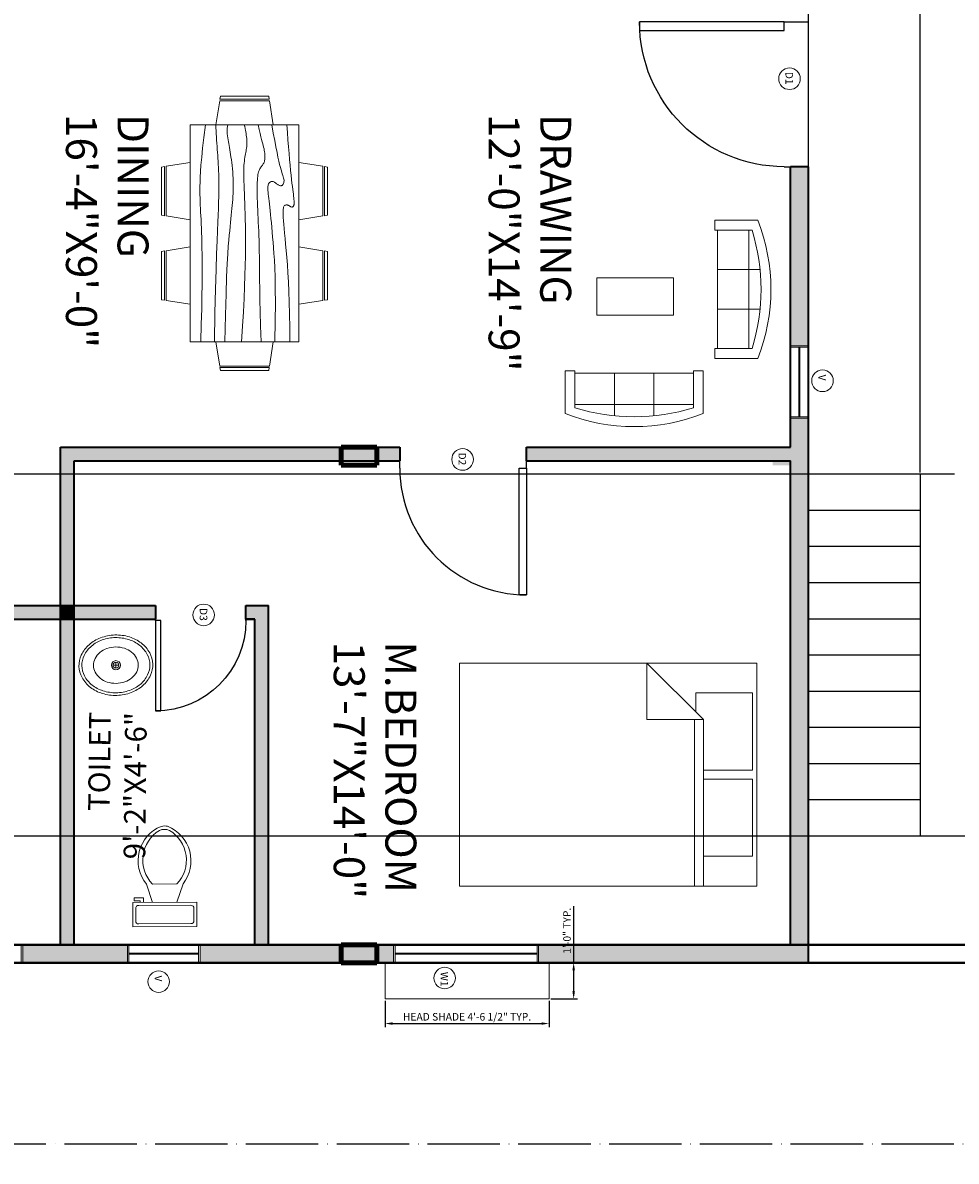
# Model space of a CAD drawing. Units: inches. Extents: x 7028582 to 7030319, y 63109697 to 63111305.
# Tile 5 of 18: x 7029402 to 7029711, y 63109901 to 63110278. Entities that reach past the tile are written whole.
import ezdxf

# ---------------------------------------------------------------- set-up
doc = ezdxf.new("R2010")
doc.units = ezdxf.units.IN
doc.linetypes.add('ACAD_ISO04W100', pattern=[30, 24, -3, 0, -3])
for name, color, linetype, lineweight in [('A-AREA-IDEN', 7, 'Continuous', 18), ('A-DOOR-IDEN', 20, 'Continuous', 13), ('A-FLOR-FIXT', 9, 'Continuous', 18), ('A-FLOR-STRS', 1, 'Continuous', 25), ('A-GLAZ-IDEN', 20, 'Continuous', 13), ('A-WALL-PATT', 8, 'Continuous', 13), ('C-ANNO-DIMS', 7, 'Continuous', 18), ('C-PROP', 1, 'ACAD_ISO04W100', 25), ('doors', 20, 'Continuous', 25), ('furniture', 9, 'Continuous', 18), ('PILLARS', 220, 'Continuous', 100), ('S-COLS-PATT', 220, 'Continuous', 100), ('walls', 6, 'Continuous', 35), ('WINDOW SHADOW', 9, 'Continuous', 13), ('windows', 5, 'Continuous', 18)]:
    doc.layers.add(name, color=color, linetype=linetype, lineweight=lineweight)
doc.styles.get("Standard").update_dxf_attribs({"font": 'arial.ttf'})
doc.dimstyles.new('ISO-25', dxfattribs={"dimtxt": 2.5, "dimasz": 2.5, "dimexe": 1.25, "dimexo": 0.625, "dimtad": 1, "dimlunit": 4, "dimtxsty": 'Standard', "dimcen": 2.5, "dimadec": 0, "dimazin": 0, "dimtfac": 1, "dimtmove": 0, "dimatfit": 3, "dimfxl": 1, "dimarcsym": 0})

# ---------------------------------------------------------------- blocks, each defined once
blk = doc.blocks.new('*U2')
for p, q in [((0, 0), (0, -5)), ((30, 0), (30, -5))]:
    blk.add_line(p, q)
blk.add_lwpolyline([(0, 0), (0, 30), (1.75, 30), (1.75, 0)], close=True)
blk.add_arc((0, 0), 30, 0, 90)
blk = doc.blocks.new('Dining Set - 36 x 72 in.')
for p, q in [((-22, 27.5), (-22.1562, 26.50042)), ((-5.8416, 26.5), (-22.1534, 26.5)), ((-22, 27.5), (-6, 27.5)), ((-5.8437, 26.49966), (-6, 27.5)), ((6, 27.5), (5.8438, 26.50042)), ((22.1584, 26.5), (5.8466, 26.5)), ((6, 27.5), (22, 27.5)), ((22.1563, 26.49966), (22, 27.5)), ((-22.2343, 26.00059), (-23.4847, 17.99762)), ((-22.2304, 26), (-5.7608, 26)), ((-4.5152, 17.99762), (-5.7655, 25.99926)), ((5.7657, 26.00059), (4.5153, 17.99762)), ((5.7696, 26), (22.2392, 26)), ((23.4848, 17.99762), (22.2345, 25.99926)), ((36, 18), (-36, 18)), ((-36, 18), (-36, -18)), ((36, -18), (36, 18)), ((-45.5, 8), (-44.5004, 8.15617)), ((-45.5, 8), (-45.5, -8)), ((-44.5, -8.15843), (-44.5, 8.15338)), ((-44.0006, 8.23428), (-35.9976, 9.48474)), ((-44, 8.23041), (-44, -8.23915)), ((44.0006, 8.23428), (35.9976, 9.48474)), ((44, 8.23041), (44, -8.23915)), ((44.5, -8.15843), (44.5, 8.15338)), ((45.5, 8), (44.5005, 8.15617)), ((45.5, 8), (45.5, -8)), ((-44.4997, -8.15631), (-45.5, -8)), ((-35.9976, -9.48476), (-43.9993, -8.2345)), ((35.9976, -9.48476), (43.9993, -8.2345)), ((44.4997, -8.15631), (45.5, -8)), ((-36, -18), (36, -18)), ((-22.2343, -26.0006), (-23.4847, -17.99762)), ((-4.5152, -17.99762), (-5.7655, -25.99928)), ((5.7657, -26.0006), (4.5153, -17.99762)), ((23.4848, -17.99762), (22.2345, -25.99928)), ((-22.2304, -26), (-5.7608, -26)), ((5.7696, -26), (22.2392, -26)), ((-22, -27.5), (-22.1562, -26.50044)), ((-5.8416, -26.5), (-22.1534, -26.5)), ((-22, -27.5), (-6, -27.5)), ((-5.8437, -26.49967), (-6, -27.5)), ((6, -27.5), (5.8438, -26.50044)), ((22.1584, -26.5), (5.8466, -26.5)), ((6, -27.5), (22, -27.5)), ((22.1563, -26.49967), (22, -27.5))]:
    blk.add_line(p, q)
for points in [[(-36, 15), (-31.1772, 14.97754), (-26.8079, 14.91406), (-22.8538, 14.81543), (-19.276, 14.6875), (-16.0362, 14.53613), (-13.0957, 14.36718), (-10.4159, 14.18652), (-7.9583, 14), (-5.6904, 13.81315), (-3.6035, 13.63021), (-1.6954, 13.45508), (0.0365, 13.29166), (1.5945, 13.14388), (2.9811, 13.01562), (4.1988, 12.9108), (5.25, 12.83333), (6.1393, 12.78613), (6.8802, 12.76823), (7.4883, 12.77767), (7.9792, 12.8125), (8.3685, 12.87077), (8.6719, 12.95052), (8.9049, 13.0498), (9.0833, 13.16666), (9.2205, 13.29899), (9.3216, 13.44401), (9.3895, 13.59879), (9.4271, 13.76041), (9.4373, 13.92594), (9.4232, 14.09245), (9.3875, 14.257), (9.3333, 14.41666), (9.2638, 14.56917), (9.1836, 14.71484), (9.0975, 14.85465), (9.0104, 14.98958), (8.9272, 15.1206), (8.8529, 15.2487), (8.7922, 15.37483), (8.75, 15.5), (8.7305, 15.62467), (8.7344, 15.74739), (8.7617, 15.86621), (8.8125, 15.97916), (8.8867, 16.08431), (8.9844, 16.17968), (9.1055, 16.26334), (9.25, 16.33333), (9.4189, 16.38802), (9.6172, 16.42708), (9.8506, 16.45052), (10.125, 16.45833), (10.4463, 16.45052), (10.8203, 16.42708), (11.2529, 16.38802), (11.75, 16.33333), (12.3184, 16.26318), (12.9694, 16.17838), (13.7151, 16.07991), (14.5677, 15.96875), (15.5395, 15.84586), (16.6426, 15.71224), (17.8893, 15.56884), (19.2917, 15.41666), (20.859, 15.25667), (22.5879, 15.08984), (24.4721, 14.91715), (26.5052, 14.73958), (28.6809, 14.5581), (30.9929, 14.3737), (33.4347, 14.18733), (36, 14)], [(-36, 10), (-28.9766, 10.14274), (-23.1725, 10.20442), (-18.4241, 10.19775), (-14.5677, 10.13541), (-11.4399, 10.03011), (-8.877, 9.89453), (-6.7154, 9.74137), (-4.7917, 9.58333), (-2.9698, 9.43082), (-1.2246, 9.28515), (0.4415, 9.14534), (2.026, 9.01041), (3.5266, 8.87939), (4.9408, 8.7513), (6.266, 8.62516), (7.5, 8.5), (8.6411, 8.37549), (9.6914, 8.2539), (10.6538, 8.13818), (11.5312, 8.03125), (12.3267, 7.93603), (13.043, 7.85547), (13.6831, 7.79248), (14.25, 7.75), (14.7471, 7.7303), (15.1797, 7.73307), (15.5537, 7.75732), (15.875, 7.80208), (16.1494, 7.86637), (16.3828, 7.94922), (16.5811, 8.04964), (16.75, 8.16666), (16.8944, 8.29915), (17.0143, 8.44531), (17.1089, 8.60319), (17.1771, 8.77083), (17.218, 8.94629), (17.2305, 9.1276), (17.2137, 9.31282), (17.1667, 9.5), (17.0895, 9.6875), (16.987, 9.875), (16.8649, 10.0625), (16.7292, 10.25), (16.5856, 10.4375), (16.4401, 10.625), (16.2985, 10.8125), (16.1667, 11), (16.05, 11.18733), (15.9518, 11.3737), (15.8752, 11.5581), (15.8229, 11.73958), (15.798, 11.91715), (15.8034, 12.08984), (15.842, 12.25667), (15.9167, 12.41666), (16.0295, 12.56836), (16.1784, 12.70833), (16.3605, 12.83268), (16.5729, 12.9375), (16.8127, 13.01888), (17.0768, 13.07291), (17.3625, 13.0957), (17.6667, 13.08333), (17.9894, 13.03312), (18.3418, 12.94726), (18.7382, 12.82918), (19.1927, 12.68229), (19.7195, 12.51001), (20.3327, 12.31575), (21.0465, 12.10294), (21.875, 11.875), (22.8357, 11.63354), (23.959, 11.37304), (25.2786, 11.08618), (26.8282, 10.76562), (28.6414, 10.40405), (30.752, 9.99414), (33.1936, 9.52856), (36, 9)], [(-36, 5.5), (-30.7157, 5.3348), (-26.069, 5.20963), (-21.9946, 5.11767), (-18.4271, 5.05208), (-15.3009, 5.00602), (-12.5508, 4.97265), (-10.1112, 4.94515), (-7.9167, 4.91666), (-5.909, 4.88167), (-4.0586, 4.83984), (-2.3429, 4.79215), (-0.7396, 4.73958), (0.7739, 4.6831), (2.22, 4.6237), (3.6213, 4.56233), (5, 4.5), (6.373, 4.43782), (7.7344, 4.3776), (9.0723, 4.32129), (10.375, 4.27083), (11.6309, 4.22819), (12.8281, 4.19531), (13.9551, 4.17415), (15, 4.16666), (15.954, 4.17448), (16.819, 4.19791), (17.6001, 4.23698), (18.3021, 4.29166), (18.9299, 4.36198), (19.4883, 4.44791), (19.9823, 4.54948), (20.4167, 4.66666), (20.7969, 4.79899), (21.1302, 4.94401), (21.4245, 5.09879), (21.6875, 5.26041), (21.9271, 5.42594), (22.1511, 5.59245), (22.3672, 5.757), (22.5834, 5.91666), (22.8065, 6.06868), (23.0404, 6.21093), (23.2879, 6.34147), (23.5521, 6.45833), (23.8358, 6.55957), (24.142, 6.64323), (24.4735, 6.70735), (24.8334, 6.75), (25.2235, 6.76969), (25.642, 6.76692), (26.0858, 6.74267), (26.5521, 6.69791), (27.0379, 6.63362), (27.5404, 6.55078), (28.0565, 6.45036), (28.5834, 6.33333), (29.1242, 6.19987), (29.7071, 6.04687), (30.3661, 5.87044), (31.1354, 5.66666), (32.0493, 5.43164), (33.142, 5.16146), (34.4475, 4.85221), (36, 4.5)], [(-36, -1), (-30.7915, -0.6591), (-26.0195, -0.38216), (-21.6519, -0.16284), (-17.6563, 0.00521), (-14.0005, 0.12833), (-10.6523, 0.21289), (-7.5796, 0.26522), (-4.75, 0.29166), (-2.134, 0.29793), (0.2878, 0.28711), (2.5317, 0.26163), (4.6146, 0.22396), (6.5529, 0.17651), (8.3633, 0.12174), (10.0623, 0.06209), (11.6667, 0), (13.1899, -0.06201), (14.6341, -0.1211), (15.9982, -0.17432), (17.2813, -0.21875), (18.4823, -0.25147), (19.6003, -0.26953), (20.6343, -0.27002), (21.5834, -0.25), (22.4481, -0.20768), (23.2357, -0.14584), (23.9549, -0.06836), (24.6146, 0.02083), (25.2235, 0.11784), (25.7904, 0.21875), (26.3241, 0.31966), (26.8334, 0.41666), (27.3265, 0.50618), (27.8099, 0.58593), (28.2894, 0.65397), (28.7709, 0.70833), (29.2601, 0.74707), (29.763, 0.76823), (30.2855, 0.76985), (30.8334, 0.75), (31.4088, 0.70784), (31.9994, 0.64713), (32.589, 0.57275), (33.1615, 0.48958), (33.7008, 0.4025), (34.1908, 0.3164), (34.6153, 0.23616), (34.9584, 0.16666), (35.2099, 0.11165), (35.3848, 0.07031), (35.504, 0.04069), (35.5886, 0.02083), (35.6594, 0.00879), (35.7377, 0.0026), (35.8442, 0.00032), (36, 0)], [(-36, -6.5), (-27.1843, -6.31267), (-20.084, -6.1263), (-14.469, -5.9419), (-10.1094, -5.76042), (-6.7752, -5.58285), (-4.2363, -5.41016), (-2.2629, -5.24333), (-0.625, -5.08334), (0.8708, -4.93099), (2.2715, -4.78646), (3.5872, -4.64974), (4.8281, -4.52084), (6.0046, -4.39974), (7.127, -4.28646), (8.2053, -4.18099), (9.25, -4.08334), (10.2705, -3.99382), (11.2734, -3.91407), (12.2647, -3.84603), (13.25, -3.79167), (14.2354, -3.75293), (15.2266, -3.73177), (16.2295, -3.73015), (17.25, -3.75), (18.2912, -3.79248), (19.3451, -3.85547), (20.4009, -3.93604), (21.4479, -4.03125), (22.4754, -4.13819), (23.4727, -4.25391), (24.4289, -4.37549), (25.3334, -4.5), (26.1785, -4.62492), (26.9694, -4.74935), (27.7145, -4.87281), (28.4219, -4.99479), (29.1, -5.11483), (29.7572, -5.23242), (30.4016, -5.34709), (31.0417, -5.45834), (31.6837, -5.56437), (32.3262, -5.65821), (32.9658, -5.73153), (33.599, -5.77604), (34.2224, -5.78345), (34.8327, -5.74545), (35.4264, -5.65373), (36, -5.5)], [(-36, -10), (-26.4022, -9.81299), (-18.4675, -9.62891), (-11.9839, -9.45069), (-6.7396, -9.28125), (-2.5226, -9.12354), (0.8789, -8.98047), (3.6769, -8.85498), (6.0833, -8.75), (8.2767, -8.66765), (10.3021, -8.60677), (12.1712, -8.56543), (13.8958, -8.54167), (15.4876, -8.53353), (16.9583, -8.53907), (18.3197, -8.55632), (19.5834, -8.58334), (20.7616, -8.61841), (21.8685, -8.66081), (22.9188, -8.71004), (23.9271, -8.76563), (24.9081, -8.82707), (25.8763, -8.89388), (26.8465, -8.96558), (27.8334, -9.04167), (28.8474, -9.12118), (29.8828, -9.20117), (30.93, -9.27824), (31.9792, -9.34896), (33.0205, -9.40991), (34.0443, -9.45768), (35.0407, -9.48885), (36, -9.5)], [(-36, -14.5), (-30.0881, -14.33513), (-25.0332, -14.21224), (-20.7312, -14.12647), (-17.0781, -14.07292), (-13.97, -14.04671), (-11.3027, -14.04297), (-8.9724, -14.05681), (-6.875, -14.08334), (-4.9224, -14.11833), (-3.0905, -14.16016), (-1.3709, -14.20785), (0.2448, -14.26042), (1.7647, -14.3169), (3.1973, -14.3763), (4.5507, -14.43767), (5.8333, -14.5), (7.0554, -14.5621), (8.235, -14.62175), (9.3922, -14.67652), (10.5469, -14.72396), (11.7192, -14.76164), (12.929, -14.78711), (14.1965, -14.79794), (15.5417, -14.79167), (16.9933, -14.76424), (18.6152, -14.70508), (20.4804, -14.60197), (22.6615, -14.44271), (25.2312, -14.21509), (28.2624, -13.9069), (31.8277, -13.50594), (36, -13)]]:
    blk.add_lwpolyline(points)
blk = doc.blocks.new('Sofa - Roundback 7 ft.')
for p, q in [((-12.00002, -32.4421), (-12.00003, -6.5971)), ((11.99997, -32.4421), (11.99998, -6.5971)), ((-36.000027, -34), (-36.000027, -11.4696)), ((-35.999844, -13.3819), (35.9998, -13.3819)), ((35.99998, -34), (35.99998, -11.4696)), ((-36.000027, -32.4421), (35.99998, -32.4421))]:
    blk.add_line(p, q)
for points in [[(-36.000027, -34), (-42.000027, -34), (-42.000027, -8)], [(41.99998, -8), (41.99998, -34), (35.99998, -34)]]:
    blk.add_lwpolyline(points)
for centre, radius, start, end in [((0, -114.25), 114.25, 68.43141, 111.5686), ((-0.00001, -127.1968), 121.1968, 72.72033, 107.2797)]:
    blk.add_arc(centre, radius, start, end)
blk = doc.blocks.new('Toilet - top')
for p, q in [((9.5, -6), (9.5, -2)), ((-10, -8.5), (-8, -8.5)), ((-10, -9.5), (-10, -8.5)), ((-7, -9.5), (-10, -9.5)), ((-8, -8.5), (-8, -8)), ((-7, -8), (-7, -9.5)), ((-4, -8), (-6, -14)), ((4, -8), (6, -14)), ((4, -14), (-4, -14))]:
    blk.add_line(p, q)
blk.add_lwpolyline([(10.5, -8), (10.5, 0), (-10.5, 0), (-10.5, -8)], close=True)
for points in [[(-9.5, -2), (-9.5, -6)], [(8.5, -1), (-8.5, -1)], [(-8.5, -7), (8.5, -7)]]:
    blk.add_lwpolyline(points)
for centre, radius, start, end in [((-8.62, -1.88), 0.884, 81.8699, 188.1301), ((8.62, -1.88), 0.884, 351.8699, 98.1301), ((-8.62, -6.12), 0.884, 171.8699, 278.1301), ((8.62, -6.12), 0.884, 261.8699, 8.1301), ((3.52, -21.58), 12.17, 141.4691, 247.9714), ((4.2, -21.82), 11.33, 136.3677, 238.9468), ((-3.52, -21.58), 12.17, 292.0284, 38.5307), ((-4.2, -21.82), 11.33, 301.053, 43.6321), ((0, -27.88), 4, 245.7318, 294.2682), ((0, -29), 4, 254.8605, 285.1395)]:
    blk.add_arc(centre, radius, start, end)
blk = doc.blocks.new('Sink - Oval top')
for p, q in [((-1, 0), (1, 0)), ((0, 1), (0, -1))]:
    blk.add_line(p, q)
for points in [[(-12.23, 0.39, 0.117634), (-11.46, -3.36, 0.104469), (-8.88, -6.8, 0.090016), (-5.08, -9.07, 0.08192), (-0.32, -10.02, 0.08192), (4.49, -9.38, 0.090016), (8.42, -7.36, 0.104469), (11.22, -4.09, 0.117634), (12.23, -0.39, 0.117634), (11.46, 3.36, 0.104469), (8.88, 6.8, 0.090016), (5.08, 9.07, 0.08192), (0.32, 10.02, 0.08192), (-4.49, 9.38, 0.090016), (-8.42, 7.36, 0.104469), (-11.22, 4.09, 0.117634)], [(-11.29, 0.16, 0.118622), (-10.52, -3.25, 0.104678), (-8.07, -6.36, 0.089562), (-4.54, -8.37, 0.081185), (-0.13, -9.15, 0.081185), (4.3, -8.49, 0.089562), (7.89, -6.58, 0.104678), (10.42, -3.55, 0.118622), (11.29, -0.16, 0.118622), (10.52, 3.25, 0.104678), (8.07, 6.36, 0.089562), (4.54, 8.37, 0.081185), (0.13, 9.15, 0.081185), (-4.3, 8.49, 0.089562), (-7.89, 6.58, 0.104678), (-10.42, 3.55, 0.118622)], [(-7.42, 0.08, 0.118283), (-6.91, -2.17, 0.104607), (-5.29, -4.21, 0.089718), (-2.97, -5.53, 0.081436), (-0.07, -6.04, 0.081436), (2.84, -5.59, 0.089718), (5.2, -4.33, 0.104607), (6.86, -2.32, 0.118283), (7.42, -0.08, 0.118283), (6.91, 2.17, 0.104607), (5.29, 4.21, 0.089718), (2.97, 5.53, 0.081436), (0.07, 6.04, 0.081436), (-2.84, 5.59, 0.089718), (-5.2, 4.33, 0.104607), (-6.86, 2.32, 0.118283)]]:
    blk.add_lwpolyline(points, format="xyb", close=True)
for radius in [1.5, 1]:
    blk.add_circle((0, 0), radius)
blk = doc.blocks.new('Bed - Queen')
for p, q in [((0, -80.00003), (0, 0)), ((0, 0), (59.99999, 0)), ((59.99999, 0), (59.99999, -80.00003)), ((7.99999, -1.2), (28.79998, -1.2)), ((7.99999, -14.4), (7.99999, -1.2)), ((28.79998, -1.2), (28.79998, -14.4)), ((31.19999, -1.2), (51.99999, -1.2)), ((31.19999, -14.4), (31.19999, -1.2)), ((51.99999, -1.2), (51.99999, -16.4)), ((0, -14.4), (44.8, -14.4)), ((59.99999, -29.6), (44.8, -14.4)), ((44.8, -14.4), (44.8, -29.6)), ((44.8, -16.8), (0, -16.8)), ((51.99999, -16.4), (46.79936, -16.4)), ((44.8, -29.6), (59.99999, -29.6)), ((59.99999, -80.00003), (0, -80.00003))]:
    blk.add_line(p, q)
blk = doc.blocks.new('WIN-SASH-24')
for p, q in [((24.05, 6), (0, 6)), ((0.5, 6), (0.5, 0)), ((23.55, 0), (23.55, 6)), ((0, 0), (24.05, 0)), ((23.55, 3.2), (0.5, 3.2)), ((23.55, 2.8), (0.5, 2.8))]:
    blk.add_line(p, q)
blk = doc.blocks.new('WIN-SASH-24-FRAME')
for p, q in [((24.05, 6), (0, 6)), ((0.5, 6), (0.5, 0)), ((23.55, 0), (23.55, 6)), ((0, 0), (24.05, 0))]:
    blk.add_line(p, q)
blk = doc.blocks.new('WIN-SASH-48')
for p, q in [((48.05, 6), (0, 6)), ((0.5, 6), (0.5, 0)), ((47.55, 0), (47.55, 6)), ((47.55, 3.2), (0.5, 3.2)), ((47.55, 2.8), (0.5, 2.8)), ((0, 0), (48.05, 0))]:
    blk.add_line(p, q)
blk = doc.blocks.new('WINDOW-SHADE-HEAD-54')
for p, q in [((0, 0), (0, 12)), ((54.39, 12), (54.39, 0)), ((54.39, 0), (0, 0))]:
    blk.add_line(p, q)
blk = doc.blocks.new('COLUMN-RECT-PROFILE')
for p, q in [((11.91, 6), (0, 6)), ((0, 6), (0, 0)), ((11.91, 0), (11.91, 6)), ((0, 0), (11.91, 0))]:
    blk.add_line(p, q)
blk = doc.blocks.new('TABLE-COFFEE-RECT')
blk.add_lwpolyline([(25.34, 12.34), (0, 12.34), (0, 0), (25.34, 0)], close=True)
blk = doc.blocks.new('TAG-D2-ST-L')
blk.add_circle((3.58, 3.58), 3.58)
blk.add_text('D2', height=2.5, rotation=270).set_placement((2.23, 5.87))
blk = doc.blocks.new('TAG-D3-ST-L')
blk.add_circle((3.58, 3.58), 3.58)
blk.add_text('D3', height=2.5, rotation=270).set_placement((2.27, 5.87))
blk = doc.blocks.new('TAG-V-ST-L')
blk.add_circle((3.58, 3.58), 3.58)
blk.add_text('V', height=2.5, rotation=270).set_placement((2.23, 5.62))
blk = doc.blocks.new('TAG-W1-ST-L')
blk.add_circle((3.58, 3.58), 3.58)
blk.add_text('W1', height=2.5, rotation=270).set_placement((2.23, 5.64))
blk = doc.blocks.new('*D93')
at = {"layer": 'C-ANNO-DIMS', "color": 0, "lineweight": -2, "transparency": 16777216}
for p, q in [((7029521.82, 63109953.93), (7029521.82, 63109945.15)), ((7029576.21, 63109953.93), (7029576.21, 63109945.15)), ((7029524.32, 63109946.4), (7029573.71, 63109946.4))]:
    blk.add_line(p, q, dxfattribs=at)
at = {"layer": 'C-ANNO-DIMS', "color": 0, "lineweight": 100, "transparency": 16777216}
for points in [[(7029524.32, 63109946.81), (7029524.32, 63109945.98), (7029521.82, 63109946.4)], [(7029573.71, 63109946.81), (7029573.71, 63109945.98), (7029576.21, 63109946.4)]]:
    blk.add_solid(points, dxfattribs=at)
at = {"layer": 'Defpoints', "color": 0, "lineweight": 100, "transparency": 16777216}
for p in [(7029521.82, 63109954.56), (7029576.21, 63109954.56), (7029576.21, 63109946.4)]:
    blk.add_point(p, dxfattribs=at)
at = {"layer": 'C-ANNO-DIMS', "color": 0, "transparency": 16777216, "insert": (7029549.01, 63109948.32), "char_height": 2.5, "attachment_point": 5}
blk.add_mtext('HEAD SHADE 4\'-6 1/2" TYP.', dxfattribs=at)
blk = doc.blocks.new('*D94')
at = {"layer": 'C-ANNO-DIMS', "color": 0, "lineweight": -2, "transparency": 16777216}
for p, q in [((7029584.37, 63109966.56), (7029584.37, 63109985.31)), ((7029576.84, 63109966.56), (7029585.62, 63109966.56)), ((7029584.37, 63109957.06), (7029584.37, 63109964.06)), ((7029576.84, 63109954.56), (7029585.62, 63109954.56))]:
    blk.add_line(p, q, dxfattribs=at)
at = {"layer": 'C-ANNO-DIMS', "color": 0, "lineweight": 100, "transparency": 16777216}
for points in [[(7029583.95, 63109964.06), (7029584.79, 63109964.06), (7029584.37, 63109966.56)], [(7029583.95, 63109957.06), (7029584.79, 63109957.06), (7029584.37, 63109954.56)]]:
    blk.add_solid(points, dxfattribs=at)
at = {"layer": 'Defpoints', "color": 0, "lineweight": 100, "transparency": 16777216}
for p in [(7029576.21, 63109966.56), (7029584.37, 63109966.56), (7029576.21, 63109954.56)]:
    blk.add_point(p, dxfattribs=at)
at = {"layer": 'C-ANNO-DIMS', "color": 0, "transparency": 16777216, "insert": (7029582.47, 63109977.18), "char_height": 2.5, "attachment_point": 5, "rotation": 90}
blk.add_mtext('1\'-0" TYP.', dxfattribs=at)
blk = doc.blocks.new('*D99')
at = {"layer": 'C-ANNO-DIMS', "color": 0, "lineweight": -2, "transparency": 16777216}
for p, q in [((7029234.71, 63109965.93), (7029234.71, 63109697.14)), ((7030175.71, 63109965.93), (7030175.71, 63109697.14)), ((7029237.21, 63109698.39), (7030173.21, 63109698.39))]:
    blk.add_line(p, q, dxfattribs=at)
at = {"layer": 'C-ANNO-DIMS', "color": 0, "lineweight": 100, "transparency": 16777216}
for points in [[(7029237.21, 63109698.8), (7029237.21, 63109697.97), (7029234.71, 63109698.39)], [(7030173.21, 63109698.8), (7030173.21, 63109697.97), (7030175.71, 63109698.39)]]:
    blk.add_solid(points, dxfattribs=at)
at = {"layer": 'Defpoints', "color": 0, "lineweight": 100, "transparency": 16777216}
for p in [(7029234.71, 63109966.56), (7030175.71, 63109966.56), (7030175.71, 63109698.39)]:
    blk.add_point(p, dxfattribs=at)
at = {"layer": 'C-ANNO-DIMS', "color": 0, "transparency": 16777216, "insert": (7029705.21, 63109700.29), "char_height": 2.5, "attachment_point": 5}
blk.add_mtext('78\'-5"', dxfattribs=at)
blk = doc.blocks.new('*D108')
at = {"layer": 'C-ANNO-DIMS', "color": 0, "lineweight": -2, "transparency": 16777216}
for p, q in [((7029662.21, 63110129.18), (7029662.21, 63111300.44)), ((7029664.71, 63111299.19), (7029696.71, 63111299.19)), ((7029699.21, 63110129.18), (7029699.21, 63111300.44))]:
    blk.add_line(p, q, dxfattribs=at)
at = {"layer": 'C-ANNO-DIMS', "color": 0, "lineweight": 100, "transparency": 16777216}
for points in [[(7029664.71, 63111299.61), (7029664.71, 63111298.77), (7029662.21, 63111299.19)], [(7029696.71, 63111299.61), (7029696.71, 63111298.77), (7029699.21, 63111299.19)]]:
    blk.add_solid(points, dxfattribs=at)
at = {"layer": 'Defpoints', "color": 0, "lineweight": 100, "transparency": 16777216}
for p in [(7029699.21, 63111299.19), (7029662.21, 63110128.56), (7029699.21, 63110128.56)]:
    blk.add_point(p, dxfattribs=at)
at = {"layer": 'C-ANNO-DIMS', "color": 0, "transparency": 16777216, "insert": (7029680.71, 63111301.09), "char_height": 2.5, "attachment_point": 5}
blk.add_mtext('3\'-1"', dxfattribs=at)
blk = doc.blocks.new('*D109')
at = {"layer": 'C-ANNO-DIMS', "color": 0, "lineweight": -2, "transparency": 16777216}
for p, q in [((7029710.58, 63110128.56), (7028586.23, 63110128.56)), ((7028587.48, 63110126.06), (7028587.48, 63110011.06)), ((7029710.58, 63110008.56), (7028586.23, 63110008.56))]:
    blk.add_line(p, q, dxfattribs=at)
at = {"layer": 'C-ANNO-DIMS', "color": 0, "lineweight": 100, "transparency": 16777216}
for points in [[(7028587.06, 63110126.06), (7028587.89, 63110126.06), (7028587.48, 63110128.56)], [(7028587.06, 63110011.06), (7028587.89, 63110011.06), (7028587.48, 63110008.56)]]:
    blk.add_solid(points, dxfattribs=at)
at = {"layer": 'Defpoints', "color": 0, "lineweight": 100, "transparency": 16777216}
for p in [(7029711.21, 63110128.56), (7028587.48, 63110008.56), (7029711.21, 63110008.56)]:
    blk.add_point(p, dxfattribs=at)
at = {"layer": 'C-ANNO-DIMS', "color": 0, "transparency": 16777216, "insert": (7028585.57, 63110068.56), "char_height": 2.5, "attachment_point": 5, "rotation": 90}
blk.add_mtext('10\'-0"', dxfattribs=at)
blk = doc.blocks.new('*D110')
at = {"layer": 'C-ANNO-DIMS', "color": 0, "lineweight": -2, "transparency": 16777216}
for p, q in [((7029747.58, 63110008.56), (7028586.23, 63110008.56)), ((7028587.48, 63110006.06), (7028587.48, 63109975.06)), ((7029747.58, 63109972.56), (7028586.23, 63109972.56))]:
    blk.add_line(p, q, dxfattribs=at)
at = {"layer": 'C-ANNO-DIMS', "color": 0, "lineweight": 100, "transparency": 16777216}
for points in [[(7028587.06, 63110006.06), (7028587.89, 63110006.06), (7028587.48, 63110008.56)], [(7028587.06, 63109975.06), (7028587.89, 63109975.06), (7028587.48, 63109972.56)]]:
    blk.add_solid(points, dxfattribs=at)
at = {"layer": 'Defpoints', "color": 0, "lineweight": 100, "transparency": 16777216}
for p in [(7029748.21, 63110008.56), (7028587.48, 63109972.56), (7029748.21, 63109972.56)]:
    blk.add_point(p, dxfattribs=at)
at = {"layer": 'C-ANNO-DIMS', "color": 0, "transparency": 16777216, "insert": (7028585.57, 63109990.56), "char_height": 2.5, "attachment_point": 5, "rotation": 90}
blk.add_mtext('3\'-0"', dxfattribs=at)

msp = doc.modelspace()

# ---------------------------------------------------------------- hatches: boundary and pattern name
at = {"layer": 'A-WALL-PATT'}
h = msp.add_hatch(color=256, dxfattribs=at)
h.dxf.hatch_style = 1
h.paths.add_polyline_path([(7029656.205, 63110230.557), (7029662.205, 63110230.557), (7029662.205, 63110171.186), (7029656.205, 63110171.186)])
h = msp.add_hatch(color=256, dxfattribs=at)
h.dxf.hatch_style = 1
h.paths.add_polyline_path([(7029568.726, 63110137.557), (7029656.205, 63110137.557), (7029656.205, 63110147.137), (7029662.205, 63110147.137), (7029662.205, 63109966.557), (7029572.732, 63109966.557), (7029572.732, 63109972.557), (7029656.205, 63109972.557), (7029656.205, 63110133.057), (7029568.726, 63110133.057)])
h = msp.add_hatch(color=256, dxfattribs=at)
h.dxf.hatch_style = 1
h.paths.add_polyline_path([(7029414.205, 63110137.557), (7029414.205, 63110085.057), (7029418.705, 63110085.057), (7029418.705, 63110133.057), (7029526.726, 63110133.057), (7029526.726, 63110137.557)])
h = msp.add_hatch(color=256, dxfattribs=at)
h.dxf.hatch_style = 1
h.paths.add_polyline_path([(7029414.205, 63110080.557), (7029414.205, 63110085.057), (7029360.705, 63110085.057), (7029360.705, 63110077.557), (7029365.205, 63110077.557), (7029365.205, 63110080.557)])
h = msp.add_hatch(color=256, dxfattribs=at)
h.dxf.hatch_style = 1
h.paths.add_polyline_path([(7029414.205, 63110085.057), (7029418.705, 63110085.057), (7029418.705, 63110080.557), (7029414.205, 63110080.557)])
h = msp.add_hatch(color=256, dxfattribs=at)
h.dxf.hatch_style = 1
h.paths.add_polyline_path([(7029418.705, 63110085.057), (7029445.705, 63110085.057), (7029445.705, 63110080.557), (7029418.705, 63110080.557)])
h = msp.add_hatch(color=256, dxfattribs=at)
h.dxf.hatch_style = 1
h.paths.add_polyline_path([(7029460.479, 63109972.557), (7029478.705, 63109972.557), (7029478.705, 63110080.557), (7029475.705, 63110080.557), (7029475.705, 63110085.057), (7029483.205, 63110085.057), (7029483.205, 63109972.557), (7029524.683, 63109972.557), (7029524.683, 63109966.557), (7029460.479, 63109966.557)])
h = msp.add_hatch(color=256, dxfattribs=at)
h.dxf.hatch_style = 1
h.paths.add_polyline_path([(7029414.205, 63110080.557), (7029414.205, 63109972.557), (7029401.714, 63109972.557), (7029401.714, 63109966.557), (7029436.431, 63109966.557), (7029436.431, 63109972.557), (7029418.705, 63109972.557), (7029418.705, 63110080.557)])
at = {"layer": 'S-COLS-PATT'}
h = msp.add_hatch(color=256, dxfattribs=at)
h.dxf.hatch_style = 1
h.paths.add_polyline_path([(7029662.205, 63110137.557), (7029650.291, 63110137.557), (7029650.291, 63110131.557), (7029662.205, 63110131.557)])
h = msp.add_hatch(color=256, dxfattribs=at)
h.dxf.hatch_style = 1
h.paths.add_polyline_path([(7029662.205, 63109972.505), (7029650.291, 63109972.505), (7029650.291, 63109966.505), (7029662.205, 63109966.505)])

# ---------------------------------------------------------------- linework, layer by layer
at = {"layer": 'A-DOOR-IDEN'}
msp.add_circle((7029655.936, 63110259.719), 3.577, dxfattribs=at)
at = {"layer": 'A-FLOR-STRS'}
for p, q in [((7029662.205, 63110128.557), (7029662.205, 63109972.557)), ((7029699.205, 63110128.557), (7029662.205, 63110128.557)), ((7029699.205, 63110128.557), (7029699.205, 63110008.557)), ((7029699.205, 63110116.557), (7029662.205, 63110116.557)), ((7029699.205, 63110104.557), (7029662.205, 63110104.557)), ((7029699.205, 63110092.557), (7029662.205, 63110092.557)), ((7029699.205, 63110080.557), (7029662.205, 63110080.557)), ((7029699.205, 63110068.557), (7029662.205, 63110068.557)), ((7029699.205, 63110056.557), (7029662.205, 63110056.557)), ((7029699.205, 63110044.557), (7029662.205, 63110044.557)), ((7029699.205, 63110032.557), (7029662.205, 63110032.557)), ((7029699.205, 63110020.557), (7029662.205, 63110020.557)), ((7029748.205, 63110008.557), (7029662.205, 63110008.557))]:
    msp.add_line(p, q, dxfattribs=at)
at = {"layer": 'C-PROP'}
msp.add_line((7029174.705, 63109906.557), (7030235.705, 63109906.557), dxfattribs=at)
at = {"layer": 'walls'}
for p, q in [((7029656.205, 63110137.557), (7029656.205, 63110230.557)), ((7029662.205, 63110230.557), (7029656.205, 63110230.557)), ((7029662.205, 63109966.557), (7029662.205, 63110230.557)), ((7029414.205, 63109972.557), (7029414.205, 63110137.557)), ((7029414.205, 63110137.557), (7029526.726, 63110137.557)), ((7029526.726, 63110137.557), (7029526.726, 63110133.057)), ((7029568.726, 63110137.557), (7029656.205, 63110137.557)), ((7029568.726, 63110133.057), (7029568.726, 63110137.557)), ((7029418.705, 63109972.557), (7029418.705, 63110133.057)), ((7029418.705, 63110133.057), (7029526.726, 63110133.057)), ((7029568.726, 63110133.057), (7029656.205, 63110133.057)), ((7029656.205, 63109972.557), (7029656.205, 63110133.057)), ((7029360.705, 63110085.057), (7029445.705, 63110085.057)), ((7029445.705, 63110085.057), (7029445.705, 63110080.557)), ((7029475.705, 63110085.057), (7029483.205, 63110085.057)), ((7029475.705, 63110080.557), (7029475.705, 63110085.057)), ((7029483.205, 63109972.557), (7029483.205, 63110085.057)), ((7029365.205, 63110080.557), (7029445.705, 63110080.557)), ((7029475.705, 63110080.557), (7029478.705, 63110080.557)), ((7029478.705, 63110080.557), (7029475.705, 63110080.557)), ((7029478.705, 63109972.557), (7029478.705, 63110080.557)), ((7029240.705, 63109972.557), (7030169.705, 63109972.557)), ((7030169.705, 63109972.557), (7029240.705, 63109972.557)), ((7029365.205, 63109972.557), (7029414.205, 63109972.557)), ((7029418.705, 63109972.557), (7029478.705, 63109972.557)), ((7029483.205, 63109972.557), (7029656.205, 63109972.557)), ((7029748.205, 63109972.557), (7029662.205, 63109972.557)), ((7029748.205, 63109972.557), (7029662.205, 63109972.557)), ((7029234.705, 63109966.557), (7030175.705, 63109966.557)), ((7030175.705, 63109966.557), (7029234.705, 63109966.557)), ((7029234.705, 63109966.557), (7029662.205, 63109966.557))]:
    msp.add_line(p, q, dxfattribs=at)
at = {"layer": 'windows'}
for p, q in [((7029656.205, 63110171.186), (7029662.205, 63110171.186)), ((7029662.205, 63110147.137), (7029656.205, 63110147.137)), ((7029401.714, 63109972.557), (7029401.714, 63109966.557)), ((7029436.431, 63109966.557), (7029436.431, 63109972.557)), ((7029460.479, 63109972.557), (7029460.479, 63109966.557)), ((7029524.683, 63109966.557), (7029524.683, 63109972.557)), ((7029572.732, 63109972.557), (7029572.732, 63109966.557))]:
    msp.add_line(p, q, dxfattribs=at)

# ---------------------------------------------------------------- block references
at = {"layer": 'A-DOOR-IDEN'}
for name, p in [('TAG-D2-ST-L', (7029543.956, 63110129.893)), ('TAG-D3-ST-L', (7029458.118, 63110078.328))]:
    msp.add_blockref(name, p, dxfattribs=at)
at = {"layer": 'A-FLOR-FIXT', "xscale": -1}
msp.add_blockref('Sink - Oval top', (7029432.582, 63110065.243), dxfattribs=at)
at = {"layer": 'A-FLOR-FIXT', "xscale": -1.013555723357934, "yscale": 1.013555723357934, "zscale": 1.013555723357934, "rotation": 180.274620379553}
msp.add_blockref('Toilet - top', (7029448.831, 63109978.497), dxfattribs=at)
at = {"layer": 'A-GLAZ-IDEN'}
for name, p in [('TAG-V-ST-L', (7029663.285, 63110155.979)), ('TAG-W1-ST-L', (7029538.009, 63109957.914)), ('TAG-V-ST-L', (7029443.2, 63109956.713))]:
    msp.add_blockref(name, p, dxfattribs=at)
at = {"layer": 'doors'}
for p, xscale, yscale, zscale, rotation in [((7029654.205, 63110278.557), -1.599999999999999, 1.599999999999999, 1.599999999999999, 90), ((7029568.726, 63110130.557), 1.399999999999999, 1.399999999999999, 1.399999999999999, 180)]:
    msp.add_blockref('*U2', p, dxfattribs=dict(at, xscale=xscale, yscale=yscale, zscale=zscale, rotation=rotation))
at = {"layer": 'doors', "xscale": -1, "rotation": 180}
msp.add_blockref('*U2', (7029445.705, 63110080.057), dxfattribs=at)
at = {"layer": 'furniture', "xscale": -1, "rotation": 270}
msp.add_blockref('Dining Set - 36 x 72 in.', (7029475.247, 63110208.448), dxfattribs=at)
at = {"layer": 'furniture'}
for name, p, xscale, yscale, zscale, rotation in [('Sofa - Roundback 7 ft.', (7029649.752, 63110189.875), -0.5455524879488546, 0.5455524879488546, 0.5455524879488546, 270), ('Sofa - Roundback 7 ft.', (7029604.428, 63110144.346), -0.5455524879488546, 0.5455524879488546, 0.5455524879488546, 180), ('Bed - Queen', (7029645.108, 63109992.002), -1.232093012797833, 1.232093012797833, 1.232093012797833, 270)]:
    msp.add_blockref(name, p, dxfattribs=dict(at, xscale=xscale, yscale=yscale, zscale=zscale, rotation=rotation))
at = {"layer": 'furniture', "extrusion": (0, 0, -1), "zscale": -1}
msp.add_blockref('TABLE-COFFEE-RECT', (-7029617.436, 63110181.346), dxfattribs=at)
at = {"layer": 'PILLARS'}
for p in [(7029507.238, 63110131.557), (7029507.238, 63109966.505)]:
    msp.add_blockref('COLUMN-RECT-PROFILE', p, dxfattribs=at)
at = {"layer": 'WINDOW SHADOW'}
msp.add_blockref('WINDOW-SHADE-HEAD-54', (7029521.817, 63109954.557), dxfattribs=at)
at = {"layer": 'windows', "rotation": 269.9999999843229}
msp.add_blockref('WIN-SASH-24', (7029656.205, 63110171.186), dxfattribs=at)
at = {"layer": 'windows'}
for name, p in [('WIN-SASH-24-FRAME', (7029377.666, 63109966.557)), ('WIN-SASH-24', (7029436.431, 63109966.557)), ('WIN-SASH-48', (7029524.683, 63109966.557))]:
    msp.add_blockref(name, p, dxfattribs=at)

# ---------------------------------------------------------------- texts
at = {"layer": 'A-AREA-IDEN'}
for s, width, gutter_width, insert, char_height, attachment_point, rotation in [('DINING\\P16\'-4"X9\'-0"', 82.04322, 51.315, (7029416.035, 63110248.03), 10.26307, 7, 270), ('DRAWING\\P12\'-0"X14\'-9"', 82.04322, 51.315, (7029556.17, 63110248.03), 10.26307, 7, 270), ('M.BEDROOM\\P13\'-7"X14\'-0"', 82.04322, 51.315, (7029504.833, 63110073.083), 10.26307, 7, 270), ('TOILET\\P9\'-2"X4\'-6"', 42.97461, 35.821, (7029423.746, 63110049.835), 7.16426, 3, 89.3536)]:
    msp.add_mtext_dynamic_manual_height_columns(s, width=width, gutter_width=gutter_width, heights=[0], dxfattribs=dict(at, insert=insert, char_height=char_height, attachment_point=attachment_point, rotation=rotation))
at = {"layer": 'A-DOOR-IDEN'}
msp.add_text('D1', height=2.5, rotation=270, dxfattribs=at).set_placement((7029654.584, 63110262.013))

# ---------------------------------------------------------------- dimensions: what is measured, and where the dimension line sits
at = {"layer": 'C-ANNO-DIMS'}
for base, p1, p2, picture, middle in [((7029699.205, 63111299.19), (7029662.205, 63110128.557), (7029699.205, 63110128.557), '*D108', (7029680.705, 63111301.092)), ((7030175.705, 63109698.385), (7029234.705, 63109966.557), (7030175.705, 63109966.557), '*D99', (7029705.205, 63109700.287))]:
    dim = msp.add_linear_dim(base=base, p1=p1, p2=p2, dimstyle='ISO-25', override={"dimdec": 1, "dimlfac": 1, "dimrnd": 0, "dimzin": 1, "dimdsep": 46, "dimlunit": 4, "dimfrac": 2}, dxfattribs=at)
    dim.commit()
    dim.dimension.update_dxf_attribs({"geometry": picture, "text_midpoint": middle})
for base, p1, p2, picture, middle in [((7028587.475, 63110008.557), (7029711.205, 63110128.557), (7029711.205, 63110008.557), '*D109', (7028585.574, 63110068.557)), ((7028587.475, 63109972.557), (7029748.205, 63110008.557), (7029748.205, 63109972.557), '*D110', (7028585.573, 63109990.557))]:
    dim = msp.add_linear_dim(base=base, p1=p1, p2=p2, angle=90, dimstyle='ISO-25', override={"dimdec": 1, "dimlfac": 1, "dimrnd": 0, "dimzin": 1, "dimdsep": 46, "dimlunit": 4, "dimfrac": 2}, dxfattribs=at)
    dim.commit()
    dim.dimension.update_dxf_attribs({"geometry": picture, "text_midpoint": middle})
dim = msp.add_linear_dim(base=(7029584.371, 63109966.557), p1=(7029576.212, 63109954.557), p2=(7029576.212, 63109966.557), angle=90, text='<> TYP.', dimstyle='ISO-25', override={"dimdec": 1, "dimlfac": 1, "dimrnd": 0, "dimzin": 1, "dimdsep": 46, "dimlunit": 4, "dimfrac": 2}, dxfattribs=at)
dim.commit()
dim.dimension.update_dxf_attribs({"geometry": '*D94', "text_midpoint": (7029582.47, 63109977.183)})
dim = msp.add_linear_dim(base=(7029576.212, 63109946.397), p1=(7029521.817, 63109954.557), p2=(7029576.212, 63109954.557), text='HEAD SHADE <> TYP.', dimstyle='ISO-25', override={"dimdec": 1, "dimlfac": 1, "dimrnd": 0, "dimzin": 1, "dimdsep": 46, "dimlunit": 4, "dimfrac": 2}, dxfattribs=at)
dim.commit()
dim.dimension.update_dxf_attribs({"geometry": '*D93', "text_midpoint": (7029549.015, 63109948.315)})

doc.saveas('drawing.dxf')
